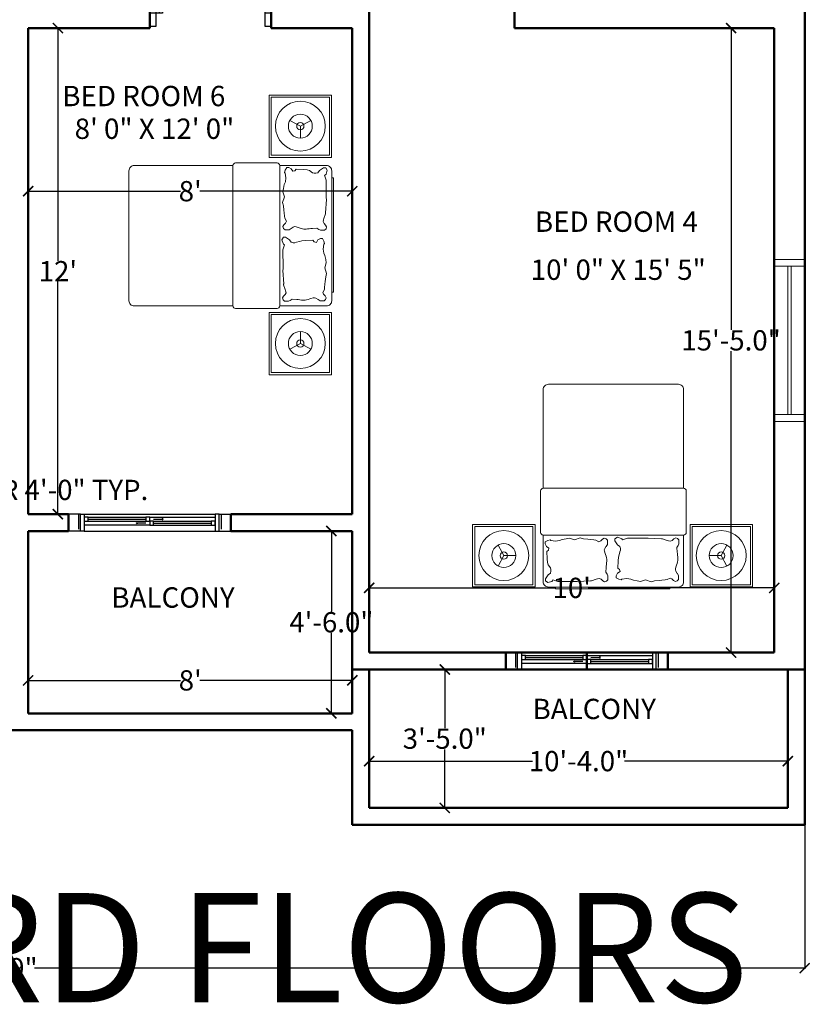
# Model space of a CAD drawing. Units: inches. Extents: x 147 to 1638, y 107 to 941.
# Tile 14 of 17: x 1362 to 1596, y 107 to 398. Entities that reach past the tile are written whole.
import ezdxf

# ---------------------------------------------------------------- set-up
doc = ezdxf.new("R2010")
doc.units = ezdxf.units.IN
doc.header["$MEASUREMENT"] = 0
for name, color, linetype, lineweight in [('A-ANNO-DIMS', 2, 'Continuous', 15), ('A-ANNO-TEXT', 7, 'Continuous', 25), ('A-AREA-IDEN', 7, 'Continuous', 18), ('A-Door', 150, 'Continuous', 25), ('furniture', 50, 'Continuous', 18), ('walls', 7, 'Continuous', 50), ('windows', 3, 'Continuous', 20)]:
    doc.layers.add(name, color=color, linetype=linetype, lineweight=lineweight)
doc.layers.add('A-Glaz', color=92, linetype='Continuous')
doc.layers.add('NT', color=1, linetype='Continuous')
doc.styles.get("Standard").update_dxf_attribs({"font": 'arial.ttf'})
doc.dimstyles.get("Standard").update_dxf_attribs({"dimtxt": 6, "dimasz": 3, "dimexe": 0.18, "dimexo": 0.0625, "dimgap": 0.09, "dimtad": 0, "dimtih": 1, "dimtoh": 1, "dimdec": 1, "dimzin": 0, "dimdsep": 46, "dimlunit": 3, "dimtxsty": 'Standard', "dimblk": 'ARCHTICK', "dimcen": 0.09, "dimadec": 0, "dimazin": 0, "dimtfac": 1, "dimtdec": 1, "dimtofl": 0, "dimtmove": 0, "dimatfit": 3, "dimfxl": 1, "dimtolj": 1, "dimtzin": 0, "dimarcsym": 0})

# ---------------------------------------------------------------- blocks, each defined once
blk = doc.blocks.new('A$C087A3AA9')
at = {"layer": 'A-Door'}
for points in [[(852.6, 94.7), (852.6, 852.6), (805.3, 852.6), (805.3, 94.7)], [(47.4, 94.7), (47.4, 0), (0, 0), (0, 94.7)], [(900, 94.7), (900, 0), (852.6, 0), (852.6, 94.7)]]:
    blk.add_lwpolyline(points, close=True, dxfattribs=at)
at = {"layer": 'A-Glaz'}
blk.add_line((828.9, 852.6), (828.9, 94.7), dxfattribs=at)
at = {"layer": 'NT'}
blk.add_arc((805.3, 94.7), 757.9, 90, 180, dxfattribs=at)
blk = doc.blocks.new('_ArchTick')
at = {"color": 0, "linetype": 'ByBlock', "const_width": 0.15}
blk.add_lwpolyline([(-0.5, -0.5), (0.5, 0.5)], dxfattribs=at)
blk = doc.blocks.new('*D36')
at = {"layer": 'A-ANNO-DIMS', "color": 0, "lineweight": -2, "transparency": 16777216}
for p, q in [((1364.77, 347.47), (1364.77, 347.59)), ((1364.77, 347.41), (1409.91, 347.41)), ((1460.77, 347.41), (1415.62, 347.41)), ((1460.77, 347.47), (1460.77, 347.59))]:
    blk.add_line(p, q, dxfattribs=at)
at = {"layer": 'Defpoints', "color": 0, "lineweight": -2, "transparency": 16777216}
for p in [(1364.77, 347.41), (1460.77, 347.41), (1460.77, 347.41)]:
    blk.add_point(p, dxfattribs=at)
at = {"layer": 'A-ANNO-DIMS', "color": 0, "lineweight": -2, "transparency": 16777216, "xscale": 3, "yscale": 3, "zscale": 3, "rotation": 180}
blk.add_blockref('_ArchTick', (1364.77, 347.41), dxfattribs=at)
at = {"layer": 'A-ANNO-DIMS', "color": 0, "lineweight": -2, "transparency": 16777216, "xscale": 3, "yscale": 3, "zscale": 3}
blk.add_blockref('_ArchTick', (1460.77, 347.41), dxfattribs=at)
at = {"layer": 'A-ANNO-DIMS', "color": 0, "transparency": 16777216, "insert": (1412.77, 347.41), "char_height": 6, "attachment_point": 5}
blk.add_mtext("\\A1;8'", dxfattribs=at)
blk = doc.blocks.new('*D37')
at = {"layer": 'A-ANNO-DIMS', "color": 0, "lineweight": -2, "transparency": 16777216}
for p, q in [((1371.76, 395.72), (1373.76, 395.72)), ((1373.58, 395.72), (1373.58, 326.82)), ((1373.58, 251.72), (1373.58, 320.62)), ((1370.83, 251.72), (1373.76, 251.72))]:
    blk.add_line(p, q, dxfattribs=at)
at = {"layer": 'Defpoints', "color": 0, "lineweight": -2, "transparency": 16777216}
for p in [(1371.7, 395.72), (1370.77, 251.72), (1373.58, 251.72)]:
    blk.add_point(p, dxfattribs=at)
at = {"layer": 'A-ANNO-DIMS', "color": 0, "lineweight": -2, "transparency": 16777216, "xscale": 3, "yscale": 3, "zscale": 3}
for p, rotation in [((1373.58, 395.72), 90), ((1373.58, 251.72), 270)]:
    blk.add_blockref('_ArchTick', p, dxfattribs=dict(at, rotation=rotation))
at = {"layer": 'A-ANNO-DIMS', "color": 0, "transparency": 16777216, "insert": (1373.58, 323.72), "char_height": 6, "attachment_point": 5}
blk.add_mtext("\\A1;12'", dxfattribs=at)
blk = doc.blocks.new('*D38')
at = {"layer": 'A-ANNO-DIMS', "color": 0, "lineweight": -2, "transparency": 16777216}
for p, q in [((1465.77, 221.48), (1465.77, 230.07)), ((1465.77, 229.89), (1520.87, 229.89)), ((1585.77, 229.89), (1530.67, 229.89)), ((1585.77, 221.48), (1585.77, 230.07))]:
    blk.add_line(p, q, dxfattribs=at)
at = {"layer": 'Defpoints', "color": 0, "lineweight": -2, "transparency": 16777216}
for p in [(1585.77, 229.89), (1465.77, 221.41), (1585.77, 221.41)]:
    blk.add_point(p, dxfattribs=at)
at = {"layer": 'A-ANNO-DIMS', "color": 0, "lineweight": -2, "transparency": 16777216, "xscale": 3, "yscale": 3, "zscale": 3, "rotation": 180}
blk.add_blockref('_ArchTick', (1465.77, 229.89), dxfattribs=at)
at = {"layer": 'A-ANNO-DIMS', "color": 0, "lineweight": -2, "transparency": 16777216, "xscale": 3, "yscale": 3, "zscale": 3}
blk.add_blockref('_ArchTick', (1585.77, 229.89), dxfattribs=at)
at = {"layer": 'A-ANNO-DIMS', "color": 0, "transparency": 16777216, "insert": (1525.77, 229.89), "char_height": 6, "attachment_point": 5}
blk.add_mtext("\\A1;10'", dxfattribs=at)
blk = doc.blocks.new('*D39')
at = {"layer": 'A-ANNO-DIMS', "color": 0, "lineweight": -2, "transparency": 16777216}
for p, q in [((1571.93, 395.72), (1573.14, 395.72)), ((1572.96, 395.72), (1572.96, 306.37)), ((1572.96, 210.72), (1572.96, 300.06)), ((1571.93, 210.72), (1573.14, 210.72))]:
    blk.add_line(p, q, dxfattribs=at)
at = {"layer": 'Defpoints', "color": 0, "lineweight": -2, "transparency": 16777216}
for p in [(1571.87, 395.72), (1571.87, 210.72), (1572.96, 210.72)]:
    blk.add_point(p, dxfattribs=at)
at = {"layer": 'A-ANNO-DIMS', "color": 0, "lineweight": -2, "transparency": 16777216, "xscale": 3, "yscale": 3, "zscale": 3}
for p, rotation in [((1572.96, 395.72), 90), ((1572.96, 210.72), 270)]:
    blk.add_blockref('_ArchTick', p, dxfattribs=dict(at, rotation=rotation))
at = {"layer": 'A-ANNO-DIMS', "color": 0, "transparency": 16777216, "insert": (1572.96, 303.22), "char_height": 6, "attachment_point": 5}
blk.add_mtext('\\A1;15\'-5.0"', dxfattribs=at)
blk = doc.blocks.new('*D65')
at = {"layer": 'A-ANNO-DIMS', "color": 0, "lineweight": -2, "transparency": 16777216}
for p, q in [((1486.73, 205.72), (1488.34, 205.72)), ((1488.16, 205.72), (1488.16, 188.37)), ((1488.16, 164.72), (1488.16, 182.06)), ((1486.73, 164.72), (1488.34, 164.72))]:
    blk.add_line(p, q, dxfattribs=at)
at = {"layer": 'Defpoints', "color": 0, "lineweight": -2, "transparency": 16777216}
for p in [(1486.67, 205.72), (1486.67, 164.72), (1488.16, 164.72)]:
    blk.add_point(p, dxfattribs=at)
at = {"layer": 'A-ANNO-DIMS', "color": 0, "lineweight": -2, "transparency": 16777216, "xscale": 3, "yscale": 3, "zscale": 3}
for p, rotation in [((1488.16, 205.72), 90), ((1488.16, 164.72), 270)]:
    blk.add_blockref('_ArchTick', p, dxfattribs=dict(at, rotation=rotation))
at = {"layer": 'A-ANNO-DIMS', "color": 0, "transparency": 16777216, "insert": (1488.16, 185.22), "char_height": 6, "attachment_point": 5}
blk.add_mtext('\\A1;3\'-5.0"', dxfattribs=at)
blk = doc.blocks.new('*D66')
at = {"layer": 'A-ANNO-DIMS', "color": 0, "lineweight": -2, "transparency": 16777216}
for p, q in [((1465.77, 174.47), (1465.77, 178.75)), ((1465.77, 178.57), (1514.16, 178.57)), ((1589.77, 178.57), (1541.38, 178.57)), ((1589.77, 174.47), (1589.77, 178.75))]:
    blk.add_line(p, q, dxfattribs=at)
at = {"layer": 'Defpoints', "color": 0, "lineweight": -2, "transparency": 16777216}
for p in [(1589.77, 178.57), (1465.77, 174.41), (1589.77, 174.41)]:
    blk.add_point(p, dxfattribs=at)
at = {"layer": 'A-ANNO-DIMS', "color": 0, "lineweight": -2, "transparency": 16777216, "xscale": 3, "yscale": 3, "zscale": 3, "rotation": 180}
blk.add_blockref('_ArchTick', (1465.77, 178.57), dxfattribs=at)
at = {"layer": 'A-ANNO-DIMS', "color": 0, "lineweight": -2, "transparency": 16777216, "xscale": 3, "yscale": 3, "zscale": 3}
blk.add_blockref('_ArchTick', (1589.77, 178.57), dxfattribs=at)
at = {"layer": 'A-ANNO-DIMS', "color": 0, "transparency": 16777216, "insert": (1527.77, 178.57), "char_height": 6, "attachment_point": 5}
blk.add_mtext('\\A1;10\'-4.0"', dxfattribs=at)
blk = doc.blocks.new('MAT-P14')
for p, q in [((-1.3369, 1.348), (-1.3369, 1.948)), ((-1.3369, 1.948), (-0.7369, 1.948)), ((-1.3169, 1.928), (-0.7569, 1.928)), ((-1.3169, 1.368), (-1.3169, 1.928)), ((-0.7569, 1.368), (-0.7569, 1.928)), ((-0.7369, 1.348), (-0.7369, 1.948)), ((0.625, 1.95), (-0.625, 1.95)), ((0.7534, 1.348), (0.7534, 1.948)), ((1.3534, 1.948), (0.7534, 1.948)), ((1.3334, 1.928), (0.7734, 1.928)), ((0.7734, 1.368), (0.7734, 1.928)), ((1.3334, 1.368), (1.3334, 1.928)), ((1.3534, 1.348), (1.3534, 1.948)), ((-1.0369, 1.648), (-1.0913, 1.7493)), ((1.0534, 1.648), (1.1078, 1.7493)), ((-1.0369, 1.648), (-1.0913, 1.5467)), ((-1.0369, 1.648), (-0.9219, 1.648)), ((1.0534, 1.648), (0.9384, 1.648)), ((1.0534, 1.648), (1.1078, 1.5467)), ((-1.3369, 1.348), (-0.7369, 1.348)), ((-1.3169, 1.368), (-0.7569, 1.368)), ((1.3534, 1.348), (0.7534, 1.348)), ((1.3334, 1.368), (0.7734, 1.368))]:
    blk.add_line(p, q)
for points in [[(-0.675, 1.45), (-0.675, 1.9, -0.414214), (-0.625, 1.95), (0.625, 1.95, -0.414214), (0.675, 1.9), (0.675, 1.45)], [(-0.675, 1, -0.414214), (-0.7, 1.025), (-0.7, 1.425, -0.414214), (-0.675, 1.45), (0.675, 1.45, -0.414214), (0.7, 1.425), (0.7, 1.025, -0.414214), (0.675, 1)], [(-0.625, 0, -0.414214), (-0.675, 0.05), (-0.675, 1), (0.675, 1), (0.675, 0.05, -0.414214), (0.625, 0)]]:
    blk.add_lwpolyline(points, format="xyb", close=True)
for points in [[(-0.6142, 1.8182), (-0.6262, 1.8377), (-0.6262, 1.8767), (-0.6142, 1.8914), (-0.5964, 1.8963), (-0.5785, 1.8865), (-0.563, 1.8719), (-0.5451, 1.8633), (-0.5157, 1.879), (-0.4966, 1.8816), (-0.4647, 1.8842), (-0.4393, 1.8868), (-0.3947, 1.892), (-0.3629, 1.8999), (-0.3094, 1.8823), (-0.2619, 1.8969), (-0.23, 1.8916), (-0.1918, 1.8838), (-0.1664, 1.8734), (-0.1282, 1.8682), (-0.0818, 1.8753), (-0.0758, 1.8802), (-0.052, 1.8753), (-0.0281, 1.8607), (-0.0281, 1.8412), (-0.0401, 1.8168), (-0.0639, 1.8022), (-0.0598, 1.781), (-0.0431, 1.7682), (-0.0463, 1.6973), (-0.0502, 1.6621), (-0.0561, 1.6397), (-0.0619, 1.6125), (-0.0678, 1.5965), (-0.0678, 1.5789), (-0.0631, 1.5599), (-0.0393, 1.5453), (-0.0147, 1.5053), (-0.0147, 1.4858), (-0.0385, 1.4711), (-0.0751, 1.4819), (-0.081, 1.4868), (-0.087, 1.4965), (-0.1344, 1.4812), (-0.3042, 1.4815), (-0.3178, 1.4815), (-0.3355, 1.4791), (-0.4636, 1.4878), (-0.4672, 1.4865), (-0.4732, 1.4863), (-0.5167, 1.5026), (-0.5299, 1.5053), (-0.5478, 1.5102), (-0.5656, 1.5015), (-0.5812, 1.4869), (-0.599, 1.4772), (-0.6169, 1.482), (-0.6288, 1.4967), (-0.6288, 1.5357), (-0.6229, 1.5503), (-0.611, 1.5698), (-0.6136, 1.6138), (-0.6149, 1.6269), (-0.6176, 1.6443), (-0.6189, 1.6595), (-0.6202, 1.6748), (-0.6202, 1.6955), (-0.6176, 1.7075), (-0.6136, 1.7227), (-0.6083, 1.7391), (-0.6043, 1.75), (-0.5976, 1.7707), (-0.5963, 1.7848), (-0.6003, 1.7979), (-0.6136, 1.8186)], [(0.0694, 1.5591), (0.0575, 1.5396), (0.0575, 1.5006), (0.0694, 1.4859), (0.0873, 1.481), (0.1052, 1.4908), (0.1207, 1.5054), (0.1386, 1.514), (0.168, 1.4983), (0.1871, 1.4957), (0.2189, 1.4931), (0.2444, 1.4905), (0.289, 1.4853), (0.3208, 1.4774), (0.3742, 1.495), (0.4218, 1.4804), (0.4536, 1.4857), (0.4918, 1.4935), (0.5173, 1.5039), (0.5555, 1.5091), (0.6019, 1.502), (0.6079, 1.4971), (0.6317, 1.502), (0.6555, 1.5166), (0.6555, 1.5361), (0.6436, 1.5605), (0.6198, 1.5751), (0.6239, 1.5963), (0.6405, 1.6091), (0.6373, 1.68), (0.6334, 1.7152), (0.6276, 1.7376), (0.6063, 1.7648), (0.6005, 1.7808), (0.6005, 1.7984), (0.6051, 1.8174), (0.6289, 1.832), (0.6536, 1.872), (0.6536, 1.8915), (0.6298, 1.9062), (0.5932, 1.8954), (0.5872, 1.8905), (0.5813, 1.8808), (0.5338, 1.8961), (0.3795, 1.8958), (0.3658, 1.8958), (0.3482, 1.8982), (0.2201, 1.8895), (0.2165, 1.8908), (0.2104, 1.891), (0.1669, 1.8747), (0.1538, 1.872), (0.1359, 1.8671), (0.118, 1.8758), (0.1025, 1.8904), (0.0846, 1.9001), (0.0667, 1.8953), (0.0548, 1.8806), (0.0548, 1.8416), (0.0608, 1.827), (0.0727, 1.8075), (0.0701, 1.7635), (0.0688, 1.7504), (0.0661, 1.733), (0.0648, 1.7178), (0.0634, 1.7025), (0.0634, 1.6818), (0.0661, 1.6698), (0.0701, 1.6546), (0.0754, 1.6382), (0.0794, 1.6273), (0.086, 1.6066), (0.0874, 1.5925), (0.0834, 1.5794), (0.0701, 1.5587)]]:
    blk.add_lwpolyline(points)
blk.add_lwpolyline([(-0.5417, 1.95), (-0.5417, 1.9665), (0.5583, 1.9665), (0.5583, 1.95)], close=True)
for centre, radius in [((-1.0369, 1.648), 0.24), ((1.0534, 1.648), 0.24), ((-1.0369, 1.648), 0.115), ((1.0534, 1.648), 0.115), ((-1.0369, 1.648), 0.035), ((1.0534, 1.648), 0.035)]:
    blk.add_circle(centre, radius)
blk = doc.blocks.new('*D85')
at = {"layer": 'A-ANNO-DIMS', "color": 0, "lineweight": -2, "transparency": 16777216}
for p, q in [((1364.77, 202.56), (1364.77, 202.67)), ((1364.77, 202.49), (1409.91, 202.49)), ((1460.77, 202.49), (1415.62, 202.49)), ((1460.77, 202.56), (1460.77, 202.67))]:
    blk.add_line(p, q, dxfattribs=at)
at = {"layer": 'Defpoints', "color": 0, "lineweight": -2, "transparency": 16777216}
for p in [(1364.77, 202.49), (1460.77, 202.49), (1460.77, 202.49)]:
    blk.add_point(p, dxfattribs=at)
at = {"layer": 'A-ANNO-DIMS', "color": 0, "lineweight": -2, "transparency": 16777216, "xscale": 3, "yscale": 3, "zscale": 3, "rotation": 180}
blk.add_blockref('_ArchTick', (1364.77, 202.49), dxfattribs=at)
at = {"layer": 'A-ANNO-DIMS', "color": 0, "lineweight": -2, "transparency": 16777216, "xscale": 3, "yscale": 3, "zscale": 3}
blk.add_blockref('_ArchTick', (1460.77, 202.49), dxfattribs=at)
at = {"layer": 'A-ANNO-DIMS', "color": 0, "transparency": 16777216, "insert": (1412.77, 202.49), "char_height": 6, "attachment_point": 5}
blk.add_mtext("\\A1;8'", dxfattribs=at)
blk = doc.blocks.new('*D86')
at = {"layer": 'A-ANNO-DIMS', "color": 0, "lineweight": -2, "transparency": 16777216}
for p, q in [((1455.3, 246.72), (1454.4, 246.72)), ((1454.58, 246.72), (1454.58, 222.87)), ((1454.58, 192.72), (1454.58, 216.56)), ((1455.3, 192.72), (1454.4, 192.72))]:
    blk.add_line(p, q, dxfattribs=at)
at = {"layer": 'Defpoints', "color": 0, "lineweight": -2, "transparency": 16777216}
for p in [(1455.36, 246.72), (1454.58, 192.72), (1455.36, 192.72)]:
    blk.add_point(p, dxfattribs=at)
at = {"layer": 'A-ANNO-DIMS', "color": 0, "lineweight": -2, "transparency": 16777216, "xscale": 3, "yscale": 3, "zscale": 3}
for p, rotation in [((1454.58, 246.72), 90), ((1454.58, 192.72), 270)]:
    blk.add_blockref('_ArchTick', p, dxfattribs=dict(at, rotation=rotation))
at = {"layer": 'A-ANNO-DIMS', "color": 0, "transparency": 16777216, "insert": (1454.58, 219.72), "char_height": 6, "attachment_point": 5}
blk.add_mtext('\\A1;4\'-6.0"', dxfattribs=at)
blk = doc.blocks.new('WIN-48IN')
for p, q in [((9, 48), (0, 48)), ((0, 48), (0, 0)), ((9, 0), (9, 48)), ((9, 46), (0, 46)), ((4, 2), (4, 46)), ((5, 2), (5, 46)), ((0, 2), (9, 2)), ((0, 0), (9, 0))]:
    blk.add_line(p, q)
blk = doc.blocks.new('DOOR-SLIDING-48IN')
for p, q in [((3.46, 5), (0, 5)), ((2.87, 5), (2.87, 0.59)), ((3.46, 0), (3.46, 5)), ((3.46, 5), (4.63, 5)), ((4.63, 5), (43.37, 5)), ((4.63, 5), (4.63, 0)), ((5.81, 4.11), (22.83, 4.11)), ((5.81, 3.52), (22.83, 3.52)), ((5.81, 2.93), (22.83, 2.93)), ((24, 4.11), (43.37, 4.11)), ((25.17, 3.52), (27.7, 3.52)), ((25.17, 2.93), (42.19, 2.93)), ((44.54, 5), (43.37, 5)), ((43.37, 5), (43.37, 0)), ((44.54, 5), (48, 5)), ((44.54, 0), (44.54, 5)), ((45.13, 5), (45.13, 0.59)), ((3.46, 0), (0, 0)), ((4.63, 0), (3.46, 0)), ((24, 1.76), (4.63, 1.76)), ((4.63, 0), (43.37, 0)), ((22.83, 2.35), (20.3, 2.35)), ((25.17, 2.35), (42.19, 2.35)), ((25.17, 1.76), (42.19, 1.76)), ((43.37, 0), (44.54, 0)), ((44.54, 0), (48, 0))]:
    blk.add_line(p, q)
for points in [[(4.63, 2.93), (5.81, 2.93), (5.81, 4.11), (4.63, 4.11)], [(22.83, 2.93), (24, 2.93), (24, 4.11), (22.83, 4.11)], [(24, 1.76), (25.17, 1.76), (25.17, 2.93), (24, 2.93)], [(28, 3.52), (27.7, 3.7), (27.7, 3.35)], [(42.19, 1.76), (43.37, 1.76), (43.37, 2.93), (42.19, 2.93)], [(20, 2.35), (20.3, 2.52), (20.3, 2.17)]]:
    blk.add_lwpolyline(points, close=True)
blk = doc.blocks.new('*D108')
at = {"layer": 'A-ANNO-DIMS', "color": 0, "lineweight": -2, "transparency": 16777216}
for p, q in [((1281.77, 251.78), (1281.77, 259.1)), ((1281.77, 258.92), (1329.77, 258.92)), ((1329.77, 251.78), (1329.77, 259.1)), ((1329.77, 258.92), (1332.77, 258.92))]:
    blk.add_line(p, q, dxfattribs=at)
at = {"layer": 'Defpoints', "color": 0, "lineweight": -2, "transparency": 16777216}
for p in [(1329.77, 258.92), (1281.77, 251.72), (1329.77, 251.72)]:
    blk.add_point(p, dxfattribs=at)
at = {"layer": 'A-ANNO-DIMS', "color": 0, "lineweight": -2, "transparency": 16777216, "xscale": 3, "yscale": 3, "zscale": 3, "rotation": 180}
blk.add_blockref('_ArchTick', (1281.77, 258.92), dxfattribs=at)
at = {"layer": 'A-ANNO-DIMS', "color": 0, "lineweight": -2, "transparency": 16777216, "xscale": 3, "yscale": 3, "zscale": 3}
blk.add_blockref('_ArchTick', (1329.77, 258.92), dxfattribs=at)
at = {"layer": 'A-ANNO-DIMS', "color": 0, "transparency": 16777216, "insert": (1367.43, 258.92), "char_height": 6, "attachment_point": 5}
blk.add_mtext('\\A1;SLIDER 4\'-0" TYP.', dxfattribs=at)
blk = doc.blocks.new('*D134')
at = {"layer": 'A-ANNO-DIMS', "color": 0, "lineweight": -2, "transparency": 16777216}
for p, q in [((1117.77, 159.66), (1117.77, 117.04)), ((1594.77, 159.66), (1594.77, 117.04)), ((1117.77, 117.22), (1345.87, 117.22)), ((1594.77, 117.22), (1366.66, 117.22))]:
    blk.add_line(p, q, dxfattribs=at)
at = {"layer": 'Defpoints', "color": 0, "lineweight": -2, "transparency": 16777216}
for p in [(1117.77, 159.72), (1594.77, 159.72), (1594.77, 117.22)]:
    blk.add_point(p, dxfattribs=at)
at = {"layer": 'A-ANNO-DIMS', "color": 0, "lineweight": -2, "transparency": 16777216, "xscale": 3, "yscale": 3, "zscale": 3, "rotation": 180}
blk.add_blockref('_ArchTick', (1117.77, 117.22), dxfattribs=at)
at = {"layer": 'A-ANNO-DIMS', "color": 0, "lineweight": -2, "transparency": 16777216, "xscale": 3, "yscale": 3, "zscale": 3}
blk.add_blockref('_ArchTick', (1594.77, 117.22), dxfattribs=at)
at = {"layer": 'A-ANNO-DIMS', "color": 0, "transparency": 16777216, "insert": (1356.27, 117.22), "char_height": 6, "attachment_point": 5}
blk.add_mtext('\\A1;39\'-9"', dxfattribs=at)

msp = doc.modelspace()

# ---------------------------------------------------------------- linework, layer by layer
at = {"layer": 'walls'}
for p, q in [((1594.77, 909.72), (1594.77, 201.72)), ((1508.77, 448.72), (1508.77, 395.72)), ((1465.77, 436.72), (1465.77, 210.72)), ((1400.77, 400.72), (1400.77, 395.72)), ((1436.77, 400.72), (1436.77, 395.72)), ((1364.77, 395.72), (1364.77, 251.72)), ((1364.77, 395.72), (1388.77, 395.72)), ((1400.77, 395.72), (1388.77, 395.72)), ((1436.77, 395.72), (1460.77, 395.72)), ((1460.77, 395.72), (1460.77, 251.72)), ((1508.77, 395.72), (1585.77, 395.72)), ((1585.77, 395.72), (1585.77, 210.72)), ((1364.77, 251.72), (1376.77, 251.72)), ((1376.77, 251.72), (1376.77, 246.72)), ((1424.77, 251.72), (1424.77, 246.72)), ((1424.77, 251.72), (1436.77, 251.72)), ((1436.77, 251.72), (1460.77, 251.72)), ((1364.77, 246.72), (1364.77, 192.72)), ((1364.77, 246.72), (1376.77, 246.72)), ((1424.77, 246.72), (1460.77, 246.72)), ((1460.77, 246.72), (1460.77, 192.72)), ((1465.77, 210.72), (1585.77, 210.72)), ((1506.27, 205.72), (1506.27, 210.72)), ((1530.27, 205.72), (1530.27, 210.72)), ((1554.27, 205.72), (1554.27, 210.72)), ((1460.77, 205.72), (1594.77, 205.72)), ((1465.77, 205.72), (1465.77, 201.72)), ((1589.77, 164.72), (1589.77, 205.72)), ((1465.77, 201.72), (1465.77, 164.72)), ((1594.77, 159.72), (1594.77, 201.72)), ((1364.77, 192.72), (1460.77, 192.72)), ((1251.77, 187.72), (1460.77, 187.72)), ((1460.77, 187.72), (1460.77, 159.72)), ((1465.77, 164.72), (1589.77, 164.72)), ((1460.77, 159.72), (1594.77, 159.72))]:
    msp.add_line(p, q, dxfattribs=at)

# ---------------------------------------------------------------- block references
at = {"layer": 'A-Door', "xscale": -0.0400000000000001, "yscale": 0.0400000000000001, "zscale": 0.0400000000000001}
msp.add_blockref('A$C087A3AA9', (1436.77, 396.32), dxfattribs=at)
at = {"layer": 'A-Door'}
for p in [(1376.77, 246.72), (1506.27, 205.72)]:
    msp.add_blockref('DOOR-SLIDING-48IN', p, dxfattribs=at)
at = {"layer": 'furniture', "yscale": 30.80045642108221, "zscale": 30.80045642108221}
for p, xscale, rotation in [((1394.63, 334.22), -30.80045642108221, 270), ((1538.11, 290.21), 30.80045642108221, 180)]:
    msp.add_blockref('MAT-P14', p, dxfattribs=dict(at, xscale=xscale, rotation=rotation))
at = {"layer": 'windows'}
msp.add_blockref('WIN-48IN', (1585.77, 279.22), dxfattribs=at)

# ---------------------------------------------------------------- texts
at = {"layer": 'A-ANNO-TEXT'}
msp.add_text('1 ST TO 3RD FLOORS', height=32.387, dxfattribs=at).set_placement((1150.48, 107.1))
at = {"layer": 'A-AREA-IDEN'}
for s, height, p in [('BED ROOM 6', 6.031, (1374.88, 372.59)), ('8\' 0" X 12\' 0"', 6.0306, (1378.54, 362.9)), ('BED ROOM 4', 6.031, (1514.86, 335.37)), ('  10\' 0" X 15\' 5"', 6.0306, (1509.93, 321.14)), ('BALCONY', 6.031, (1389.4, 224.03)), ('BALCONY', 6.031, (1514.16, 191.01))]:
    msp.add_text(s, height=height, dxfattribs=at).set_placement(p)

# ---------------------------------------------------------------- dimensions: what is measured, and where the dimension line sits
at = {"layer": 'A-ANNO-DIMS'}
for base, p1, p2, picture, middle in [((1373.58, 251.72), (1371.7, 395.72), (1370.77, 251.72), '*D37', (1373.58, 323.72)), ((1572.96, 210.72), (1571.87, 395.72), (1571.87, 210.72), '*D39', (1572.96, 303.22)), ((1454.58, 192.72), (1455.36, 246.72), (1455.36, 192.72), '*D86', (1454.58, 219.72)), ((1488.16, 164.72), (1486.67, 205.72), (1486.67, 164.72), '*D65', (1488.16, 185.22))]:
    dim = msp.add_linear_dim(base=base, p1=p1, p2=p2, angle=90, dimstyle='Standard', override={"dimclrd": 0, "dimclre": 0, "dimclrt": 0}, dxfattribs=at)
    dim.commit()
    dim.dimension.update_dxf_attribs({"geometry": picture, "text_midpoint": middle})
for base, p1, p2, override, picture, middle in [((1460.77, 347.41), (1364.77, 347.41), (1460.77, 347.41), {"dimclrd": 0, "dimclre": 0, "dimclrt": 0}, '*D36', (1412.77, 347.41)), ((1585.77, 229.89), (1465.77, 221.41), (1585.77, 221.41), {"dimclrd": 0, "dimclre": 0, "dimclrt": 0}, '*D38', (1525.77, 229.89)), ((1460.77, 202.49), (1364.77, 202.49), (1460.77, 202.49), {"dimclrd": 0, "dimclre": 0, "dimclrt": 0}, '*D85', (1412.77, 202.49)), ((1589.77, 178.57), (1465.77, 174.41), (1589.77, 174.41), {"dimclrd": 0, "dimclre": 0, "dimclrt": 0}, '*D66', (1527.77, 178.57)), ((1594.77, 117.22), (1117.77, 159.72), (1594.77, 159.72), {"dimdec": 1, "dimlfac": 1, "dimrnd": 0, "dimzin": 1, "dimdsep": 46, "dimlunit": 4, "dimfrac": 2}, '*D134', (1356.27, 117.22))]:
    dim = msp.add_linear_dim(base=base, p1=p1, p2=p2, dimstyle='Standard', override=override, dxfattribs=at)
    dim.commit()
    dim.dimension.update_dxf_attribs({"geometry": picture, "text_midpoint": middle})
dim = msp.add_linear_dim(base=(1329.77, 258.92), p1=(1281.77, 251.72), p2=(1329.77, 251.72), text='SLIDER <> TYP.', dimstyle='Standard', override={"dimdec": 1, "dimlfac": 1, "dimrnd": 0, "dimzin": 1, "dimdsep": 46, "dimlunit": 4, "dimfrac": 2}, dxfattribs=at)
dim.commit()
dim.dimension.update_dxf_attribs({"geometry": '*D108', "text_midpoint": (1367.43, 258.92)})

doc.saveas('drawing.dxf')
